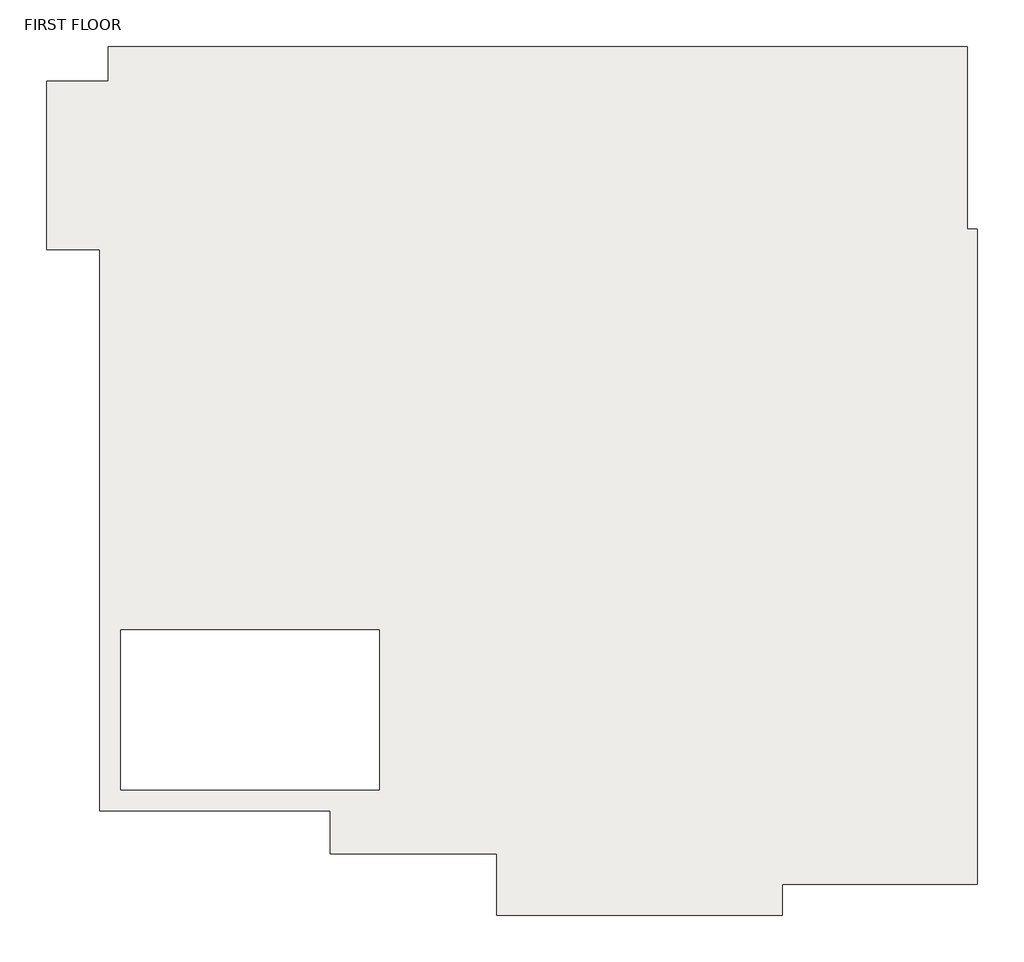
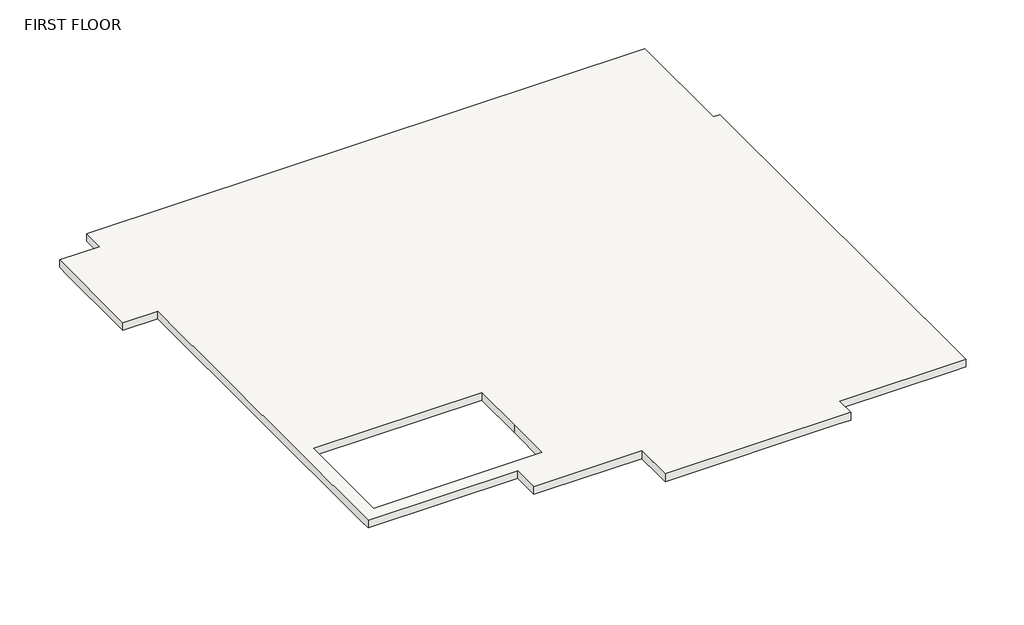
# One storey: 1 slab.
"""IFC4 building model written with IfcOpenShell, lengths in millimetres."""

from ifc_helpers import new_model, si_unit, origin, place, context, project, spatial, faceted_brep, element, save

model = new_model("IFC4")

# Units and contexts
model_context = context("Model", 3, world=origin())
ifc_project = project(units=[si_unit("LENGTHUNIT", "METRE", prefix="MILLI")], contexts=[model_context])

# Site, building, storey
site = spatial("IfcSite", under=ifc_project)
building = spatial("IfcBuilding", under=site)
storey = spatial("IfcBuildingStorey", under=building, Name="FIRST FLOOR", Elevation=3200.4)

# Slab
placement = place(None, origin())
element("IfcSlab", 1, ObjectType="2' 6", at=placement, inside=storey, context=model_context, shape_type="Brep", body=[
    faceted_brep([(2032.5798932, 5848.7877014, 3048.0), (2032.5798932, 3588.1877014, 3048.0), (2159.5798932, 3588.1877014, 3048.0), (2159.5798932, 3054.7877014, 3048.0), (2159.5798932, 2800.7877014, 3048.0), (2159.5798932, -4514.4122986, 3048.0), (1905.5798932, -4514.4122986, 3048.0), (-253.4201068, -4514.4122986, 3048.0), (-253.4201068, -4895.4122986, 3048.0), (-507.4201068, -4895.4122986, 3048.0), (-3784.0201068, -4895.4122986, 3048.0), (-3784.0201068, -4641.4122986, 3048.0), (-3784.0201068, -4133.4122986, 3048.0), (-5587.4201068, -4133.4122986, 3048.0), (-5841.4201068, -4133.4122986, 3048.0), (-5841.4201068, -3600.0122986, 3048.0), (-8686.2201068, -3600.0122986, 3048.0), (-8686.2201068, -3346.0122986, 3048.0), (-8686.2201068, 3334.1877014, 3048.0), (-9346.6201068, 3334.1877014, 3048.0), (-9346.6201068, 3588.1877014, 3048.0), (-9346.6201068, 5162.9877014, 3048.0), (-9346.6201068, 5416.9877014, 3048.0), (-8584.6201068, 5416.9877014, 3048.0), (-8584.6201068, 5848.7877014, 3048.0), (-8330.6201068, 5848.7877014, 3048.0), (-7594.0201068, 5848.7877014, 3048.0), (-7340.0201068, 5848.7877014, 3048.0), (-4317.4201068, 5848.7877014, 3048.0), (-4063.4201068, 5848.7877014, 3048.0), (-2260.0201068, 5848.7877014, 3048.0), (-2082.2201068, 5848.7877014, 3048.0), (1778.5798932, 5848.7877014, 3048.0), (-5231.8201068, -2431.6122986, 3048.0), (-5231.8201068, -1364.8122986, 3048.0), (-8432.2201068, -1364.8122986, 3048.0), (-8432.2201068, -3346.0122986, 3048.0), (-5841.4201068, -3346.0122986, 3048.0), (-5587.4201068, -3346.0122986, 3048.0), (-5231.8201068, -3346.0122986, 3048.0), (2032.5798932, 3588.1877014, 3200.4), (2032.5798932, 5848.7877014, 3200.4), (-8584.6201068, 5848.7877014, 3200.4), (-8584.6201068, 5416.9877014, 3200.4), (-9346.6201068, 5416.9877014, 3200.4), (-9346.6201068, 3334.1877014, 3200.4), (-8686.2201068, 3334.1877014, 3200.4), (-8686.2201068, -3600.0122986, 3200.4), (-5841.4201068, -3600.0122986, 3200.4), (-5841.4201068, -4133.4122986, 3200.4), (-3784.0201068, -4133.4122986, 3200.4), (-3784.0201068, -4895.4122986, 3200.4), (-253.4201068, -4895.4122986, 3200.4), (-253.4201068, -4514.4122986, 3200.4), (2159.5798932, -4514.4122986, 3200.4), (2159.5798932, 3588.1877014, 3200.4), (-5231.8201068, -1364.8122986, 3200.4), (-5231.8201068, -2431.6122986, 3200.4), (-5231.8201068, -3346.0122986, 3200.4), (-8432.2201068, -3346.0122986, 3200.4), (-8432.2201068, -1364.8122986, 3200.4)], [[[0, 1, 2, 3, 4, 5, 6, 7, 8, 9, 10, 11, 12, 13, 14, 15, 16, 17, 18, 19, 20, 21, 22, 23, 24, 25, 26, 27, 28, 29, 30, 31, 32], [33, 34, 35, 36, 37, 38, 39]], [[40, 41, 42, 43, 44, 45, 46, 47, 48, 49, 50, 51, 52, 53, 54, 55], [56, 57, 58, 59, 60]], [[1, 0, 41, 40]], [[2, 1, 40, 55]], [[5, 4, 3, 2, 55, 54]], [[7, 6, 5, 54, 53]], [[8, 7, 53, 52]], [[10, 9, 8, 52, 51]], [[12, 11, 10, 51, 50]], [[14, 13, 12, 50, 49]], [[15, 14, 49, 48]], [[16, 15, 48, 47]], [[18, 17, 16, 47, 46]], [[19, 18, 46, 45]], [[22, 21, 20, 19, 45, 44]], [[23, 22, 44, 43]], [[24, 23, 43, 42]], [[0, 32, 31, 30, 29, 28, 27, 26, 25, 24, 42, 41]], [[33, 57, 56, 34]], [[34, 56, 60, 35]], [[35, 60, 59, 36]], [[36, 59, 58, 39, 38, 37]], [[57, 33, 39, 58]]]),
])

save(model, "model.ifc")

# Revit data of these elements
# Type "2' 6"
#   Assembly Code = "B1010"
#   Function = 0
#   Layers, outside or top first: 0' - 6" "0 floor" (function 1)
# Element 1 (IfcSlab, "2' 6")
#   Height Offset From Level = 0' - 0"
#   Phase Created = New Construction
#   Materials on its faces: "0 floor"
# Materials
#   "0 floor": class "Generic", colour RGB 120 120 120, transparency 0, Cost = 0
